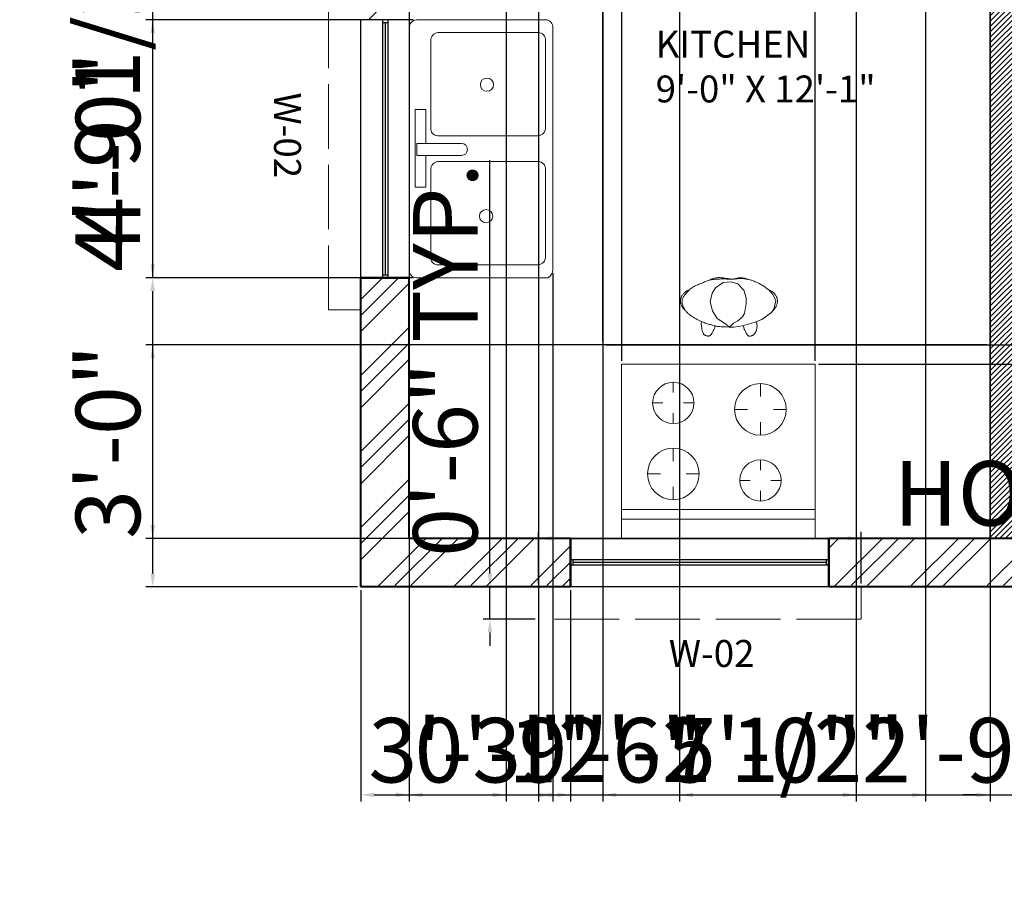
# Model space of a CAD drawing. Units: inches. Extents: x 2386 to 3029, y 792 to 1465.
# Tile 1 of 12: x 2408 to 2591, y 792 to 953. Entities that reach past the tile are written whole.
import ezdxf

# ---------------------------------------------------------------- set-up
doc = ezdxf.new("R2010")
doc.units = ezdxf.units.IN
doc.linetypes.add('ACAD_ISO02W100', pattern=[15, 12, -3])
for name, color, linetype, lineweight in [('A-AREA-IDEN', 4, 'Continuous', 25), ('A-DIMS', 1, 'Continuous', 18), ('A-EQPM', 8, 'Continuous', 18), ('A-FLOR-CASE', 6, 'Continuous', 18), ('A-FLOR-FIXT', 9, 'Continuous', 18), ('A-FURN-ENTG', 8, 'Continuous', 13), ('A-TEXT', 4, 'Continuous', 25), ('A-WALL-EXT', 7, 'Continuous', 40), ('A-WALL-INT', 9, 'Continuous', 30), ('A-WALL-PATT', 9, 'Continuous', 13), ('A-WINDOW', 4, 'Continuous', 25), ('A-WINDOW-OVHD', 4, 'ACAD_ISO02W100', 18)]:
    doc.layers.add(name, color=color, linetype=linetype, lineweight=lineweight)
doc.styles.add('ATT', font='romans.shx')
doc.styles.get("Standard").update_dxf_attribs({"font": 'arial.ttf'})
doc.dimstyles.new('ISO-25', dxfattribs={"dimtxt": 12, "dimasz": 2.5, "dimexe": 1.25, "dimexo": 0.625, "dimtad": 1, "dimlunit": 4, "dimtxsty": 'Standard', "dimcen": 2.5, "dimadec": 0, "dimazin": 0, "dimtfac": 1, "dimtmove": 0, "dimatfit": 3, "dimfxl": 1, "dimarcsym": 0})

# ---------------------------------------------------------------- blocks, each defined once
blk = doc.blocks.new('11PRNG01')
at = {"color": 0, "linetype": 'ByBlock'}
for p, q in [((0, 30), (27, 30)), ((0, 0), (0, 30)), ((3, 0), (3, 30)), ((4.5, 0), (4.5, 30)), ((27, 30), (27, 0)), ((10, 26), (10, 24)), ((21, 25.2), (21, 23.6)), ((6, 22), (8, 22)), ((14, 22), (12, 22)), ((17.8, 22), (19.4, 22)), ((24.2, 22), (22.6, 22)), ((10, 18), (10, 20)), ((21, 18.8), (21, 20.4)), ((20, 12.5), (20, 10.5)), ((9, 11.7), (9, 10.1)), ((5.8, 8.5), (7.4, 8.5)), ((12.2, 8.5), (10.6, 8.5)), ((16, 8.5), (18, 8.5)), ((24, 8.5), (22, 8.5)), ((9, 5.3), (9, 6.9)), ((20, 4.5), (20, 6.5)), ((27, 0), (0, 0))]:
    blk.add_line(p, q, dxfattribs=at)
for centre, radius in [((10, 22), 4), ((21, 22), 3.2), ((20, 8.5), 4), ((9, 8.5), 3.2)]:
    blk.add_circle(centre, radius, dxfattribs=at)
at = {"color": 0, "linetype": 'ByBlock', "style": 'ATT'}
for tag, p, flags in [('ITEM', (0, -11), 3), ('ROOM_NUMBER', (0, -20), 1), ('DEPTH', (0, -29), 3), ('WIDTH', (0, -38), 3)]:
    blk.add_attdef(tag, p, '', height=6, dxfattribs=dict(at, flags=flags))
blk = doc.blocks.new('PERSON-STANDING-PLAN')
for p, q in [((2.26, 9.11), (2.39, 9.19)), ((2.39, 9.19), (2.54, 9.27)), ((2.54, 9.27), (2.7, 9.35)), ((2.7, 9.35), (2.86, 9.42)), ((2.86, 9.42), (3.04, 9.5)), ((3.04, 9.5), (3.21, 9.57)), ((3.21, 9.57), (3.39, 9.65)), ((3.39, 9.65), (3.58, 9.72)), ((3.58, 9.72), (3.76, 9.79)), ((3.76, 9.79), (3.94, 9.87)), ((3.94, 9.87), (4.11, 9.95)), ((4.11, 9.95), (4.28, 10.02)), ((4.28, 10.02), (4.45, 10.1)), ((4.45, 10.1), (4.62, 10.18)), ((4.62, 10.18), (4.79, 10.25)), ((4.79, 10.25), (4.96, 10.31)), ((4.96, 10.31), (5.14, 10.38)), ((5.14, 10.38), (5.33, 10.43)), ((5.33, 10.43), (5.53, 10.48)), ((5.48, 10.5), (5.36, 10.44)), ((5.69, 10.59), (5.48, 10.5)), ((5.53, 10.48), (5.74, 10.51)), ((5.91, 10.67), (5.69, 10.59)), ((5.74, 10.51), (5.95, 10.55)), ((6.13, 10.74), (5.91, 10.67)), ((5.95, 10.55), (6.17, 10.57)), ((6.35, 10.79), (6.13, 10.74)), ((6.17, 10.57), (6.39, 10.59)), ((6.57, 10.84), (6.35, 10.79)), ((6.39, 10.59), (6.61, 10.61)), ((7.91, 9.98), (6.48, 9.01)), ((6.79, 10.87), (6.57, 10.84)), ((6.61, 10.61), (6.83, 10.62)), ((6.99, 10.89), (6.79, 10.87)), ((6.83, 10.62), (7.05, 10.63)), ((7.18, 10.9), (6.99, 10.89)), ((7.05, 10.63), (7.26, 10.64)), ((7.38, 10.9), (7.18, 10.9)), ((7.26, 10.64), (7.47, 10.65)), ((7.57, 10.88), (7.38, 10.9)), ((7.47, 10.65), (7.68, 10.65)), ((7.78, 10.87), (7.57, 10.88)), ((7.68, 10.65), (7.87, 10.65)), ((7.99, 10.84), (7.78, 10.87)), ((7.87, 10.65), (8.06, 10.65)), ((9.39, 10.13), (7.91, 9.98)), ((8.22, 10.82), (7.99, 10.84)), ((8.06, 10.65), (8.23, 10.65)), ((9.71, 10.64), (8.22, 10.82)), ((8.23, 10.65), (8.39, 10.65)), ((8.39, 10.65), (8.54, 10.64)), ((8.54, 10.64), (8.67, 10.64)), ((8.67, 10.64), (8.78, 10.63)), ((8.78, 10.63), (8.89, 10.62)), ((8.89, 10.62), (8.98, 10.61)), ((8.98, 10.61), (9.08, 10.6)), ((9.08, 10.6), (9.16, 10.59)), ((9.16, 10.59), (9.25, 10.59)), ((9.25, 10.59), (9.35, 10.59)), ((9.35, 10.59), (9.44, 10.59)), ((10.63, 9.72), (9.39, 10.13)), ((9.44, 10.59), (9.55, 10.6)), ((9.55, 10.6), (9.66, 10.61)), ((9.9, 10.69), (9.56, 10.61)), ((9.66, 10.61), (9.78, 10.62)), ((9.78, 10.62), (9.9, 10.63)), ((10.22, 10.76), (9.9, 10.69)), ((9.9, 10.63), (10.03, 10.64)), ((10.03, 10.64), (10.16, 10.66)), ((10.16, 10.66), (10.3, 10.67)), ((10.5, 10.81), (10.22, 10.76)), ((10.3, 10.67), (10.45, 10.68)), ((10.45, 10.68), (10.61, 10.7)), ((10.76, 10.84), (10.5, 10.81)), ((10.61, 10.7), (10.76, 10.71)), ((11.79, 8.58), (10.63, 9.72)), ((10.99, 10.86), (10.76, 10.84)), ((10.76, 10.71), (10.92, 10.71)), ((10.92, 10.71), (11.09, 10.72)), ((11.2, 10.87), (10.99, 10.86)), ((11.09, 10.72), (11.25, 10.72)), ((11.4, 10.86), (11.2, 10.87)), ((11.25, 10.72), (11.41, 10.72)), ((11.58, 10.84), (11.4, 10.86)), ((11.41, 10.72), (11.57, 10.71)), ((11.57, 10.71), (11.73, 10.7)), ((11.76, 10.81), (11.58, 10.84)), ((11.73, 10.7), (11.89, 10.68)), ((11.93, 10.77), (11.76, 10.81)), ((11.89, 10.68), (12.04, 10.67)), ((12.11, 10.73), (11.93, 10.77)), ((12.04, 10.67), (12.19, 10.64)), ((12.29, 10.67), (12.11, 10.73)), ((12.19, 10.64), (12.34, 10.62)), ((12.48, 10.61), (12.29, 10.67)), ((12.34, 10.62), (12.48, 10.59)), ((12.68, 10.55), (12.48, 10.61)), ((12.48, 10.59), (12.63, 10.56)), ((12.63, 10.56), (12.77, 10.53)), ((12.91, 10.49), (12.68, 10.55)), ((12.77, 10.53), (12.91, 10.49)), ((12.91, 10.49), (13.05, 10.45)), ((13.17, 10.43), (12.91, 10.49)), ((13.05, 10.45), (13.2, 10.41)), ((13.2, 10.41), (13.35, 10.36)), ((13.35, 10.36), (13.51, 10.3)), ((13.51, 10.3), (13.69, 10.22)), ((13.69, 10.22), (13.89, 10.14)), ((13.89, 10.14), (14.11, 10.04)), ((14.11, 10.04), (14.35, 9.93)), ((14.35, 9.93), (14.61, 9.79)), ((14.61, 9.79), (14.89, 9.64)), ((14.89, 9.64), (15.18, 9.47)), ((15.18, 9.47), (15.49, 9.28)), ((15.49, 9.28), (15.8, 9.07)), ((0.15, 7.32), (0.11, 7.23)), ((0.2, 7.42), (0.15, 7.32)), ((0.25, 7.51), (0.2, 7.42)), ((0.32, 7.61), (0.25, 7.51)), ((0.39, 7.71), (0.32, 7.61)), ((0.48, 7.82), (0.39, 7.71)), ((0.57, 7.92), (0.48, 7.82)), ((0.52, 7.3), (0.6, 7.41)), ((0.67, 8.02), (0.57, 7.92)), ((0.6, 7.41), (0.68, 7.53)), ((0.77, 8.12), (0.67, 8.02)), ((0.68, 7.53), (0.76, 7.64)), ((0.76, 7.64), (0.85, 7.75)), ((0.87, 8.21), (0.77, 8.12)), ((0.85, 7.75), (0.94, 7.85)), ((0.97, 8.29), (0.87, 8.21)), ((0.94, 7.85), (1.03, 7.96)), ((1.08, 8.36), (0.97, 8.29)), ((1.03, 7.96), (1.12, 8.07)), ((1.17, 8.42), (1.08, 8.36)), ((1.12, 8.07), (1.21, 8.17)), ((1.26, 8.47), (1.17, 8.42)), ((1.21, 8.17), (1.3, 8.27)), ((1.35, 8.51), (1.26, 8.47)), ((1.3, 8.27), (1.39, 8.37)), ((1.43, 8.54), (1.35, 8.51)), ((1.39, 8.37), (1.49, 8.47)), ((1.49, 8.56), (1.43, 8.54)), ((1.55, 8.58), (1.49, 8.56)), ((1.49, 8.47), (1.59, 8.57)), ((1.59, 8.59), (1.55, 8.58)), ((1.59, 8.57), (1.69, 8.66)), ((1.62, 8.6), (1.59, 8.59)), ((1.69, 8.66), (1.79, 8.76)), ((1.79, 8.76), (1.9, 8.85)), ((1.9, 8.85), (2.01, 8.94)), ((2.01, 8.94), (2.13, 9.02)), ((2.13, 9.02), (2.26, 9.11)), ((5.88, 8.02), (5.48, 6.38)), ((6.48, 9.01), (5.88, 8.02)), ((12.18, 7.14), (11.79, 8.58)), ((15.8, 9.07), (16.12, 8.84)), ((16.12, 8.84), (16.44, 8.59)), ((16.26, 8.74), (17.17, 7.78)), ((16.44, 8.59), (16.61, 8.53)), ((16.61, 8.53), (16.77, 8.45)), ((16.77, 8.45), (16.94, 8.35)), ((16.94, 8.35), (17.1, 8.23)), ((17.1, 8.23), (17.25, 8.1)), ((17.17, 7.78), (17.68, 6.58)), ((17.25, 8.1), (17.38, 7.96)), ((17.38, 7.96), (17.51, 7.82)), ((17.51, 7.82), (17.61, 7.69)), ((17.61, 7.69), (17.7, 7.56)), ((17.7, 7.56), (17.78, 7.45)), ((17.78, 7.45), (17.84, 7.34)), ((17.84, 7.34), (17.88, 7.24)), ((0.01, 6.79), (0, 6.7)), ((0, 6.7), (0, 6.61)), ((0, 6.61), (0, 6.52)), ((0, 6.52), (0, 6.42)), ((0, 6.42), (0.01, 6.33)), ((0.02, 6.88), (0.01, 6.79)), ((0.01, 6.33), (0.02, 6.22)), ((0.04, 6.97), (0.02, 6.88)), ((0.02, 6.22), (0.04, 6.12)), ((0.06, 7.06), (0.04, 6.97)), ((0.04, 6.12), (0.06, 6)), ((0.08, 7.15), (0.06, 7.06)), ((0.06, 6), (0.1, 5.88)), ((0.11, 7.23), (0.08, 7.15)), ((0.1, 5.88), (0.15, 5.75)), ((0.15, 5.75), (0.23, 5.6)), ((0.23, 5.6), (0.33, 5.43)), ((0.28, 6.52), (0.29, 6.66)), ((0.29, 6.38), (0.28, 6.52)), ((0.29, 6.66), (0.31, 6.8)), ((0.3, 6.24), (0.29, 6.38)), ((0.32, 6.09), (0.3, 6.24)), ((0.31, 6.8), (0.35, 6.93)), ((0.35, 5.95), (0.32, 6.09)), ((0.35, 6.93), (0.4, 7.06)), ((0.39, 5.81), (0.35, 5.95)), ((0.43, 5.68), (0.39, 5.81)), ((0.4, 7.06), (0.46, 7.18)), ((0.48, 5.55), (0.43, 5.68)), ((0.46, 7.18), (0.52, 7.3)), ((0.53, 5.42), (0.48, 5.55)), ((5.48, 6.38), (5.95, 4.72)), ((11.9, 4.25), (12.22, 6.07)), ((12.22, 6.07), (12.18, 7.14)), ((17.68, 6.58), (17.36, 5.01)), ((17.78, 5.6), (17.68, 5.42)), ((17.86, 5.75), (17.78, 5.6)), ((17.91, 5.88), (17.86, 5.75)), ((17.88, 7.24), (17.92, 7.15)), ((17.94, 6), (17.91, 5.88)), ((17.92, 7.15), (17.95, 7.06)), ((17.96, 6.12), (17.94, 6)), ((17.95, 7.06), (17.97, 6.97)), ((17.98, 6.22), (17.96, 6.12)), ((17.97, 6.97), (17.98, 6.88)), ((17.98, 6.88), (17.99, 6.79)), ((17.99, 6.33), (17.98, 6.22)), ((17.99, 6.79), (18, 6.7)), ((18, 6.42), (17.99, 6.33)), ((18, 6.7), (18.01, 6.61)), ((18.01, 6.52), (18, 6.42)), ((18.01, 6.61), (18.01, 6.52)), ((0.33, 5.43), (0.48, 5.23)), ((0.48, 5.23), (0.67, 5.01)), ((0.58, 5.3), (0.53, 5.42)), ((0.64, 5.19), (0.58, 5.3)), ((0.7, 5.07), (0.64, 5.19)), ((0.67, 5.01), (0.91, 4.75)), ((0.77, 4.96), (0.7, 5.07)), ((0.85, 4.85), (0.77, 4.96)), ((0.93, 4.74), (0.85, 4.85)), ((1.01, 4.63), (0.93, 4.74)), ((1.1, 4.52), (1.01, 4.63)), ((1.21, 4.41), (1.1, 4.52)), ((1.32, 4.3), (1.21, 4.41)), ((1.44, 4.19), (1.32, 4.3)), ((1.57, 4.08), (1.44, 4.19)), ((1.72, 3.96), (1.57, 4.08)), ((1.88, 3.84), (1.72, 3.96)), ((2.06, 3.71), (1.88, 3.84)), ((2.26, 3.59), (2.06, 3.71)), ((5.95, 4.72), (6.81, 3.29)), ((11.44, 3.53), (11.9, 4.25)), ((16.88, 4.4), (15.08, 3.08)), ((17.36, 5.01), (16.88, 4.4)), ((17.37, 5), (17.14, 4.74)), ((17.54, 5.23), (17.37, 5)), ((17.68, 5.42), (17.54, 5.23)), ((2.46, 3.46), (2.26, 3.59)), ((2.67, 3.34), (2.46, 3.46)), ((2.89, 3.21), (2.67, 3.34)), ((3.11, 3.09), (2.89, 3.21)), ((3.33, 2.98), (3.11, 3.09)), ((3.56, 2.87), (3.33, 2.98)), ((3.77, 2.77), (3.56, 2.87)), ((3.99, 2.68), (3.77, 2.77)), ((3.86, 2.7), (3.84, 2.5)), ((3.84, 2.5), (3.84, 2.27)), ((3.84, 2.27), (3.86, 2.03)), ((3.86, 2.03), (3.89, 1.79)), ((4.2, 2.6), (3.99, 2.68)), ((4.4, 2.52), (4.2, 2.6)), ((4.6, 2.45), (4.4, 2.52)), ((4.8, 2.38), (4.6, 2.45)), ((5, 2.32), (4.8, 2.38)), ((5.19, 2.26), (5, 2.32)), ((5.38, 2.2), (5.19, 2.26)), ((5.56, 2.15), (5.38, 2.2)), ((5.74, 2.09), (5.56, 2.15)), ((5.92, 2.05), (5.74, 2.09)), ((6.09, 2), (5.92, 2.05)), ((6.25, 1.96), (6.09, 2)), ((6.41, 1.92), (6.25, 1.96)), ((6.36, 1.65), (6.46, 1.91)), ((6.55, 1.89), (6.41, 1.92)), ((6.7, 1.86), (6.55, 1.89)), ((6.85, 1.83), (6.7, 1.86)), ((6.81, 3.29), (8.17, 2.41)), ((7.04, 1.81), (6.85, 1.83)), ((8.17, 2.41), (9.1, 1.71)), ((9.1, 1.71), (9.82, 2.41)), ((9.82, 2.41), (10.66, 2.88)), ((11.53, 1.95), (9.89, 1.71)), ((10.66, 2.88), (11.44, 3.53)), ((13.68, 2.54), (11.53, 1.95)), ((11.63, 1.91), (11.75, 1.61)), ((15.08, 3.08), (13.68, 2.54)), ((14.17, 2.51), (14.14, 2.7)), ((14.19, 2.34), (14.17, 2.51)), ((14.2, 2.16), (14.19, 2.34)), ((14.21, 1.99), (14.2, 2.16)), ((14.2, 1.68), (14.21, 1.83)), ((14.21, 1.83), (14.21, 1.99)), ((3.89, 1.79), (3.93, 1.54)), ((3.93, 1.54), (3.98, 1.3)), ((3.98, 1.3), (4.03, 1.08)), ((4.03, 1.08), (4.09, 0.89)), ((4.09, 0.89), (4.14, 0.73)), ((4.14, 0.73), (4.19, 0.59)), ((4.19, 0.59), (4.24, 0.49)), ((4.24, 0.49), (4.29, 0.4)), ((4.29, 0.4), (4.34, 0.34)), ((4.34, 0.34), (4.39, 0.28)), ((4.39, 0.28), (4.45, 0.24)), ((4.45, 0.24), (4.51, 0.2)), ((4.51, 0.2), (4.57, 0.17)), ((4.57, 0.17), (4.64, 0.14)), ((4.64, 0.14), (4.72, 0.11)), ((4.72, 0.11), (4.79, 0.09)), ((4.79, 0.09), (4.86, 0.07)), ((4.86, 0.07), (4.93, 0.05)), ((4.93, 0.05), (5, 0.04)), ((5, 0.04), (5.07, 0.03)), ((5.07, 0.03), (5.13, 0.03)), ((5.13, 0.03), (5.19, 0.03)), ((5.19, 0.03), (5.24, 0.03)), ((5.24, 0.03), (5.29, 0.04)), ((5.29, 0.04), (5.34, 0.05)), ((5.34, 0.05), (5.39, 0.06)), ((5.39, 0.06), (5.43, 0.08)), ((5.43, 0.08), (5.47, 0.11)), ((5.47, 0.11), (5.51, 0.13)), ((5.51, 0.13), (5.55, 0.16)), ((5.55, 0.16), (5.59, 0.2)), ((5.59, 0.2), (5.63, 0.24)), ((5.63, 0.24), (5.68, 0.29)), ((5.68, 0.29), (5.72, 0.35)), ((5.72, 0.35), (5.77, 0.42)), ((5.77, 0.42), (5.82, 0.5)), ((5.82, 0.5), (5.88, 0.59)), ((5.88, 0.59), (5.94, 0.7)), ((5.94, 0.7), (6.01, 0.83)), ((6.01, 0.83), (6.09, 0.99)), ((6.09, 0.99), (6.17, 1.17)), ((6.17, 1.17), (6.26, 1.39)), ((6.26, 1.39), (6.36, 1.65)), ((7.27, 1.79), (7.04, 1.81)), ((7.57, 1.77), (7.27, 1.79)), ((7.97, 1.75), (7.57, 1.77)), ((8.47, 1.73), (7.97, 1.75)), ((9.1, 1.71), (8.47, 1.73)), ((9.89, 1.71), (9.1, 1.71)), ((11.75, 1.61), (11.85, 1.34)), ((11.85, 1.34), (11.95, 1.1)), ((11.95, 1.1), (12.05, 0.89)), ((12.05, 0.89), (12.13, 0.71)), ((12.13, 0.71), (12.22, 0.55)), ((12.22, 0.55), (12.29, 0.41)), ((12.29, 0.41), (12.37, 0.3)), ((12.37, 0.3), (12.44, 0.21)), ((12.44, 0.21), (12.51, 0.14)), ((12.51, 0.14), (12.58, 0.08)), ((12.58, 0.08), (12.64, 0.04)), ((12.64, 0.04), (12.71, 0.02)), ((12.71, 0.02), (12.77, 0)), ((12.77, 0), (12.84, 0)), ((12.84, 0), (12.9, 0)), ((12.9, 0), (12.97, 0.01)), ((12.97, 0.01), (13.03, 0.02)), ((13.03, 0.02), (13.1, 0.04)), ((13.1, 0.04), (13.17, 0.06)), ((13.17, 0.06), (13.24, 0.09)), ((13.24, 0.09), (13.3, 0.12)), ((13.3, 0.12), (13.37, 0.15)), ((13.37, 0.15), (13.43, 0.18)), ((13.43, 0.18), (13.49, 0.22)), ((13.49, 0.22), (13.55, 0.26)), ((13.55, 0.26), (13.61, 0.31)), ((13.61, 0.31), (13.67, 0.35)), ((13.67, 0.35), (13.72, 0.41)), ((13.72, 0.41), (13.77, 0.47)), ((13.77, 0.47), (13.82, 0.53)), ((13.82, 0.53), (13.87, 0.6)), ((13.87, 0.6), (13.92, 0.67)), ((13.92, 0.67), (13.96, 0.75)), ((13.96, 0.75), (14.01, 0.84)), ((14.01, 0.84), (14.05, 0.94)), ((14.05, 0.94), (14.08, 1.04)), ((14.08, 1.04), (14.12, 1.15)), ((14.12, 1.15), (14.14, 1.27)), ((14.14, 1.27), (14.17, 1.4)), ((14.17, 1.4), (14.19, 1.54)), ((14.19, 1.54), (14.2, 1.68))]:
    blk.add_line(p, q)
blk = doc.blocks.new('WINDOW-48IN')
for p, q in [((0, 9), (48, 9)), ((0, 0), (0, 9)), ((48, 9), (48, 0)), ((48, 5), (0, 5)), ((48, 4), (0, 4)), ((0.5, 4), (0.5, 5)), ((47.5, 4.5), (0.5, 4.5)), ((47.5, 5), (47.5, 4)), ((48, 0), (0, 0))]:
    blk.add_line(p, q)
blk = doc.blocks.new('WINDOW-HOOD-48IN')
for p, q in [((0, 0), (0, 6)), ((60, 6), (60, 0)), ((60, 0), (0, 0))]:
    blk.add_line(p, q)
blk = doc.blocks.new('*D42')
at = {"layer": 'A-DIMS', "color": 0, "lineweight": -2, "transparency": 16777216}
for p, q in [((2504.19, 848.57), (2504.19, 858.2)), ((2506.69, 856.95), (2561.69, 856.95)), ((2564.19, 848.57), (2564.19, 858.2)), ((2564.19, 856.95), (2740.1, 856.95))]:
    blk.add_line(p, q, dxfattribs=at)
at = {"layer": 'A-DIMS', "color": 0, "transparency": 16777216}
for points in [[(2506.69, 857.36), (2506.69, 856.53), (2504.19, 856.95)], [(2561.69, 857.36), (2561.69, 856.53), (2564.19, 856.95)]]:
    blk.add_solid(points, dxfattribs=at)
at = {"layer": 'Defpoints', "color": 0, "transparency": 16777216}
for p in [(2564.19, 856.95), (2504.19, 847.95), (2564.19, 847.95)]:
    blk.add_point(p, dxfattribs=at)
at = {"layer": 'A-DIMS', "color": 0, "transparency": 16777216, "insert": (2653.39, 863.78), "char_height": 12, "attachment_point": 5}
blk.add_mtext('HOOD W-02 5\'-0" TYP.', dxfattribs=at)
blk = doc.blocks.new('*D43')
at = {"layer": 'A-DIMS', "color": 0, "lineweight": -2, "transparency": 16777216}
for p, q in [((2495.19, 850.45), (2495.19, 927.34)), ((2503.57, 847.95), (2493.94, 847.95)), ((2495.19, 841.95), (2495.19, 847.95)), ((2503.57, 841.95), (2493.94, 841.95)), ((2495.19, 839.45), (2495.19, 836.95))]:
    blk.add_line(p, q, dxfattribs=at)
at = {"layer": 'A-DIMS', "color": 0, "transparency": 16777216}
for points in [[(2494.77, 850.45), (2495.61, 850.45), (2495.19, 847.95)], [(2494.77, 839.45), (2495.61, 839.45), (2495.19, 841.95)]]:
    blk.add_solid(points, dxfattribs=at)
at = {"layer": 'Defpoints', "color": 0, "transparency": 16777216}
for p in [(2495.19, 847.95), (2504.19, 847.95), (2504.19, 841.95)]:
    blk.add_point(p, dxfattribs=at)
at = {"layer": 'A-DIMS', "color": 0, "transparency": 16777216, "insert": (2488.44, 890.15), "char_height": 12, "attachment_point": 5, "rotation": 90}
blk.add_mtext('0\'-6" TYP.', dxfattribs=at)
blk = doc.blocks.new('*D60')
at = {"layer": 'A-DIMS', "color": 0, "lineweight": -2, "transparency": 16777216}
for p, q in [((2471.19, 847.32), (2471.19, 808)), ((2510.19, 847.32), (2510.19, 808)), ((2473.69, 809.25), (2507.69, 809.25))]:
    blk.add_line(p, q, dxfattribs=at)
at = {"layer": 'A-DIMS', "color": 0, "transparency": 16777216}
for points in [[(2473.69, 809.66), (2473.69, 808.83), (2471.19, 809.25)], [(2507.69, 809.66), (2507.69, 808.83), (2510.19, 809.25)]]:
    blk.add_solid(points, dxfattribs=at)
at = {"layer": 'Defpoints', "color": 0, "transparency": 16777216}
for p in [(2471.19, 847.95), (2510.19, 847.95), (2510.19, 809.25)]:
    blk.add_point(p, dxfattribs=at)
at = {"layer": 'A-DIMS', "color": 0, "transparency": 16777216, "insert": (2490.69, 816), "char_height": 12, "attachment_point": 5}
blk.add_mtext('3\'-3"', dxfattribs=at)
blk = doc.blocks.new('*D61')
at = {"layer": 'A-DIMS', "color": 0, "lineweight": -2, "transparency": 16777216}
for p, q in [((2432.49, 905.45), (2432.49, 969.54)), ((2470.57, 905.45), (2431.24, 905.45)), ((2432.49, 850.45), (2432.49, 902.95)), ((2470.57, 847.95), (2431.24, 847.95))]:
    blk.add_line(p, q, dxfattribs=at)
at = {"layer": 'A-DIMS', "color": 0, "transparency": 16777216}
for points in [[(2432.07, 902.95), (2432.91, 902.95), (2432.49, 905.45)], [(2432.07, 850.45), (2432.91, 850.45), (2432.49, 847.95)]]:
    blk.add_solid(points, dxfattribs=at)
at = {"layer": 'Defpoints', "color": 0, "transparency": 16777216}
for p in [(2432.49, 905.45), (2471.19, 905.45), (2471.19, 847.95)]:
    blk.add_point(p, dxfattribs=at)
at = {"layer": 'A-DIMS', "color": 0, "transparency": 16777216, "insert": (2425.66, 938.74), "char_height": 12, "attachment_point": 5, "rotation": 90}
blk.add_mtext('4\'-9 1/2"', dxfattribs=at)
blk = doc.blocks.new('*D71')
at = {"layer": 'A-DIMS', "color": 0, "lineweight": -2, "transparency": 16777216}
for p, q in [((2480.19, 856.32), (2480.19, 808)), ((2471.19, 847.32), (2471.19, 808)), ((2473.69, 809.25), (2477.69, 809.25)), ((2480.19, 809.25), (2515.84, 809.25))]:
    blk.add_line(p, q, dxfattribs=at)
at = {"layer": 'A-DIMS', "color": 0, "transparency": 16777216}
for points in [[(2473.69, 809.66), (2473.69, 808.83), (2471.19, 809.25)], [(2477.69, 809.66), (2477.69, 808.83), (2480.19, 809.25)]]:
    blk.add_solid(points, dxfattribs=at)
at = {"layer": 'Defpoints', "color": 0, "transparency": 16777216}
for p in [(2480.19, 856.95), (2471.19, 847.95), (2480.19, 809.25)]:
    blk.add_point(p, dxfattribs=at)
at = {"layer": 'A-DIMS', "color": 0, "transparency": 16777216, "insert": (2499.26, 816), "char_height": 12, "attachment_point": 5}
blk.add_mtext('0\'-9"', dxfattribs=at)
blk = doc.blocks.new('*D72')
at = {"layer": 'A-DIMS', "color": 0, "lineweight": -2, "transparency": 16777216}
for p, q in [((2588.19, 856.32), (2588.19, 808)), ((2594.19, 847.32), (2594.19, 808)), ((2585.69, 809.25), (2583.19, 809.25)), ((2588.19, 809.25), (2594.19, 809.25)), ((2596.69, 809.25), (2632.34, 809.25))]:
    blk.add_line(p, q, dxfattribs=at)
at = {"layer": 'A-DIMS', "color": 0, "transparency": 16777216}
for points in [[(2585.69, 809.66), (2585.69, 808.83), (2588.19, 809.25)], [(2596.69, 809.66), (2596.69, 808.83), (2594.19, 809.25)]]:
    blk.add_solid(points, dxfattribs=at)
at = {"layer": 'Defpoints', "color": 0, "transparency": 16777216}
for p in [(2588.19, 856.95), (2594.19, 847.95), (2594.19, 809.25)]:
    blk.add_point(p, dxfattribs=at)
at = {"layer": 'A-DIMS', "color": 0, "transparency": 16777216, "insert": (2615.76, 816), "char_height": 12, "attachment_point": 5}
blk.add_mtext('0\'-6"', dxfattribs=at)
blk = doc.blocks.new('*D73')
at = {"layer": 'A-DIMS', "color": 0, "lineweight": -2, "transparency": 16777216}
for p, q in [((2519.68, 889.97), (2519.68, 1427.9)), ((2555.68, 889.97), (2555.68, 1427.9)), ((2522.18, 1426.65), (2553.18, 1426.65))]:
    blk.add_line(p, q, dxfattribs=at)
at = {"layer": 'A-DIMS', "color": 0, "transparency": 16777216}
for points in [[(2522.18, 1427.06), (2522.18, 1426.23), (2519.68, 1426.65)], [(2553.18, 1427.06), (2553.18, 1426.23), (2555.68, 1426.65)]]:
    blk.add_solid(points, dxfattribs=at)
at = {"layer": 'Defpoints', "color": 0, "transparency": 16777216}
for p in [(2555.68, 1426.65), (2519.68, 889.35), (2555.68, 889.35)]:
    blk.add_point(p, dxfattribs=at)
at = {"layer": 'A-DIMS', "color": 0, "transparency": 16777216, "insert": (2537.68, 1433.4), "char_height": 12, "attachment_point": 5}
blk.add_mtext('3\'-0"', dxfattribs=at)
blk = doc.blocks.new('*D74')
at = {"layer": 'A-DIMS', "color": 0, "lineweight": -2, "transparency": 16777216}
for p, q in [((2556.3, 889.35), (2931.14, 889.35)), ((2929.89, 886.85), (2929.89, 859.45)), ((2556.3, 856.95), (2931.14, 856.95)), ((2929.89, 856.95), (2929.89, 793.13))]:
    blk.add_line(p, q, dxfattribs=at)
at = {"layer": 'A-DIMS', "color": 0, "transparency": 16777216}
for points in [[(2929.47, 886.85), (2930.31, 886.85), (2929.89, 889.35)], [(2929.47, 859.45), (2930.31, 859.45), (2929.89, 856.95)]]:
    blk.add_solid(points, dxfattribs=at)
at = {"layer": 'Defpoints', "color": 0, "transparency": 16777216}
for p in [(2555.68, 889.35), (2555.68, 856.95), (2929.89, 856.95)]:
    blk.add_point(p, dxfattribs=at)
at = {"layer": 'A-DIMS', "color": 0, "transparency": 16777216, "insert": (2923.06, 823.79), "char_height": 12, "attachment_point": 5, "rotation": 90}
blk.add_mtext('2\'-8 1/2"', dxfattribs=at)
blk = doc.blocks.new('*D76')
at = {"layer": 'A-DIMS', "color": 0, "lineweight": -2, "transparency": 16777216}
for p, q in [((2480.19, 1174.77), (2480.19, 808)), ((2498.19, 1174.77), (2498.19, 808)), ((2482.69, 809.25), (2495.69, 809.25)), ((2498.19, 809.25), (2532.71, 809.25))]:
    blk.add_line(p, q, dxfattribs=at)
at = {"layer": 'A-DIMS', "color": 0, "transparency": 16777216}
for points in [[(2482.69, 809.66), (2482.69, 808.83), (2480.19, 809.25)], [(2495.69, 809.66), (2495.69, 808.83), (2498.19, 809.25)]]:
    blk.add_solid(points, dxfattribs=at)
at = {"layer": 'Defpoints', "color": 0, "transparency": 16777216}
for p in [(2480.19, 1175.39), (2498.19, 1175.39), (2498.19, 809.25)]:
    blk.add_point(p, dxfattribs=at)
at = {"layer": 'A-DIMS', "color": 0, "transparency": 16777216, "insert": (2516.7, 816), "char_height": 12, "attachment_point": 5}
blk.add_mtext('1\'-6"', dxfattribs=at)
blk = doc.blocks.new('*D77')
at = {"layer": 'A-DIMS', "color": 0, "lineweight": -2, "transparency": 16777216}
for p, q in [((2516.19, 1103.32), (2516.19, 808)), ((2576.19, 1103.32), (2576.19, 808)), ((2518.69, 809.25), (2573.69, 809.25))]:
    blk.add_line(p, q, dxfattribs=at)
at = {"layer": 'A-DIMS', "color": 0, "transparency": 16777216}
for points in [[(2518.69, 809.66), (2518.69, 808.83), (2516.19, 809.25)], [(2573.69, 809.66), (2573.69, 808.83), (2576.19, 809.25)]]:
    blk.add_solid(points, dxfattribs=at)
at = {"layer": 'Defpoints', "color": 0, "transparency": 16777216}
for p in [(2516.19, 1103.95), (2576.19, 1103.95), (2576.19, 809.25)]:
    blk.add_point(p, dxfattribs=at)
at = {"layer": 'A-DIMS', "color": 0, "transparency": 16777216, "insert": (2546.19, 816), "char_height": 12, "attachment_point": 5}
blk.add_mtext('5\'-0"', dxfattribs=at)
blk = doc.blocks.new('*D94')
at = {"layer": 'A-DIMS', "color": 0, "lineweight": -2, "transparency": 16777216}
for p, q in [((2504.19, 1205.32), (2504.19, 808)), ((2588.19, 1205.32), (2588.19, 808)), ((2506.69, 809.25), (2585.69, 809.25))]:
    blk.add_line(p, q, dxfattribs=at)
at = {"layer": 'A-DIMS', "color": 0, "transparency": 16777216}
for points in [[(2506.69, 809.66), (2506.69, 808.83), (2504.19, 809.25)], [(2585.69, 809.66), (2585.69, 808.83), (2588.19, 809.25)]]:
    blk.add_solid(points, dxfattribs=at)
at = {"layer": 'Defpoints', "color": 0, "transparency": 16777216}
for p in [(2504.19, 1205.95), (2588.19, 1205.95), (2588.19, 809.25)]:
    blk.add_point(p, dxfattribs=at)
at = {"layer": 'A-DIMS', "color": 0, "transparency": 16777216, "insert": (2546.19, 816), "char_height": 12, "attachment_point": 5}
blk.add_mtext('7\'-0"', dxfattribs=at)
blk = doc.blocks.new('*D96')
at = {"layer": 'A-DIMS', "color": 0, "lineweight": -2, "transparency": 16777216}
for p, q in [((2516.19, 893.57), (2516.19, 1427.9)), ((2588.19, 893.57), (2588.19, 1427.9)), ((2518.69, 1426.65), (2585.69, 1426.65))]:
    blk.add_line(p, q, dxfattribs=at)
at = {"layer": 'A-DIMS', "color": 0, "transparency": 16777216}
for points in [[(2518.69, 1427.06), (2518.69, 1426.23), (2516.19, 1426.65)], [(2585.69, 1427.06), (2585.69, 1426.23), (2588.19, 1426.65)]]:
    blk.add_solid(points, dxfattribs=at)
at = {"layer": 'Defpoints', "color": 0, "transparency": 16777216}
for p in [(2588.19, 1426.65), (2516.19, 892.95), (2588.19, 892.95)]:
    blk.add_point(p, dxfattribs=at)
at = {"layer": 'A-DIMS', "color": 0, "transparency": 16777216, "insert": (2552.19, 1433.4), "char_height": 12, "attachment_point": 5}
blk.add_mtext('6\'-0"', dxfattribs=at)
blk = doc.blocks.new('*D97')
at = {"layer": 'A-DIMS', "color": 0, "lineweight": -2, "transparency": 16777216}
for p, q in [((2516.82, 965.95), (2931.14, 965.95)), ((2929.89, 895.45), (2929.89, 963.45)), ((2516.82, 892.95), (2931.14, 892.95))]:
    blk.add_line(p, q, dxfattribs=at)
at = {"layer": 'A-DIMS', "color": 0, "transparency": 16777216}
for points in [[(2929.47, 963.45), (2930.31, 963.45), (2929.89, 965.95)], [(2929.47, 895.45), (2930.31, 895.45), (2929.89, 892.95)]]:
    blk.add_solid(points, dxfattribs=at)
at = {"layer": 'Defpoints', "color": 0, "transparency": 16777216}
for p in [(2516.19, 965.95), (2929.89, 965.95), (2516.19, 892.95)]:
    blk.add_point(p, dxfattribs=at)
at = {"layer": 'A-DIMS', "color": 0, "transparency": 16777216, "insert": (2923.14, 929.45), "char_height": 12, "attachment_point": 5, "rotation": 90}
blk.add_mtext('6\'-1"', dxfattribs=at)
blk = doc.blocks.new('*D98')
at = {"layer": 'A-DIMS', "color": 0, "lineweight": -2, "transparency": 16777216}
for p, q in [((2587.57, 892.95), (2431.24, 892.95)), ((2432.49, 859.45), (2432.49, 890.45)), ((2587.57, 856.95), (2431.24, 856.95))]:
    blk.add_line(p, q, dxfattribs=at)
at = {"layer": 'A-DIMS', "color": 0, "transparency": 16777216}
for points in [[(2432.07, 890.45), (2432.91, 890.45), (2432.49, 892.95)], [(2432.07, 859.45), (2432.91, 859.45), (2432.49, 856.95)]]:
    blk.add_solid(points, dxfattribs=at)
at = {"layer": 'Defpoints', "color": 0, "transparency": 16777216}
for p in [(2432.49, 892.95), (2588.19, 892.95), (2588.19, 856.95)]:
    blk.add_point(p, dxfattribs=at)
at = {"layer": 'A-DIMS', "color": 0, "transparency": 16777216, "insert": (2425.73, 874.95), "char_height": 12, "attachment_point": 5, "rotation": 90}
blk.add_mtext('3\'-0"', dxfattribs=at)
blk = doc.blocks.new('*D99')
at = {"layer": 'A-DIMS', "color": 0, "lineweight": -2, "transparency": 16777216}
for p, q in [((2530.41, 1210.29), (2530.41, 808)), ((2563.26, 1210.63), (2563.26, 808)), ((2532.91, 809.25), (2560.76, 809.25)), ((2563.26, 809.25), (2599.11, 809.25))]:
    blk.add_line(p, q, dxfattribs=at)
at = {"layer": 'A-DIMS', "color": 0, "transparency": 16777216}
for points in [[(2532.91, 809.66), (2532.91, 808.83), (2530.41, 809.25)], [(2560.76, 809.66), (2560.76, 808.83), (2563.26, 809.25)]]:
    blk.add_solid(points, dxfattribs=at)
at = {"layer": 'Defpoints', "color": 0, "transparency": 16777216}
for p in [(2530.41, 1210.91), (2563.26, 1211.26), (2563.26, 809.25)]:
    blk.add_point(p, dxfattribs=at)
at = {"layer": 'A-DIMS', "color": 0, "transparency": 16777216, "insert": (2582.43, 816), "char_height": 12, "attachment_point": 5}
blk.add_mtext('2\'-9"', dxfattribs=at)
blk = doc.blocks.new('*D102')
at = {"layer": 'A-DIMS', "color": 0, "lineweight": -2, "transparency": 16777216}
for p, q in [((2480.19, 906.32), (2480.19, 808)), ((2506.86, 906.32), (2506.86, 808)), ((2482.69, 809.25), (2504.36, 809.25)), ((2506.86, 809.25), (2570.67, 809.25))]:
    blk.add_line(p, q, dxfattribs=at)
at = {"layer": 'A-DIMS', "color": 0, "transparency": 16777216}
for points in [[(2482.69, 809.66), (2482.69, 808.83), (2480.19, 809.25)], [(2504.36, 809.66), (2504.36, 808.83), (2506.86, 809.25)]]:
    blk.add_solid(points, dxfattribs=at)
at = {"layer": 'Defpoints', "color": 0, "transparency": 16777216}
for p in [(2480.19, 906.95), (2506.86, 906.95), (2506.86, 809.25)]:
    blk.add_point(p, dxfattribs=at)
at = {"layer": 'A-DIMS', "color": 0, "transparency": 16777216, "insert": (2540.01, 816.08), "char_height": 12, "attachment_point": 5}
blk.add_mtext('2\'-2 1/2"', dxfattribs=at)
blk = doc.blocks.new('*D103')
at = {"layer": 'A-DIMS', "color": 0, "lineweight": -2, "transparency": 16777216}
for p, q in [((2480.9, 953.44), (2431.24, 953.44)), ((2432.49, 907.94), (2432.49, 950.94)), ((2480.9, 905.44), (2431.24, 905.44))]:
    blk.add_line(p, q, dxfattribs=at)
at = {"layer": 'A-DIMS', "color": 0, "transparency": 16777216}
for points in [[(2432.07, 950.94), (2432.91, 950.94), (2432.49, 953.44)], [(2432.07, 907.94), (2432.91, 907.94), (2432.49, 905.44)]]:
    blk.add_solid(points, dxfattribs=at)
at = {"layer": 'Defpoints', "color": 0, "transparency": 16777216}
for p in [(2432.49, 953.44), (2481.52, 953.44), (2481.52, 905.44)]:
    blk.add_point(p, dxfattribs=at)
at = {"layer": 'A-DIMS', "color": 0, "transparency": 16777216, "insert": (2425.74, 929.44), "char_height": 12, "attachment_point": 5, "rotation": 90}
blk.add_mtext('4\'-0"', dxfattribs=at)

msp = doc.modelspace()

# ---------------------------------------------------------------- hatches: boundary and pattern name
at = {"layer": 'A-WALL-PATT'}
h = msp.add_hatch(dxfattribs=at)
h.set_pattern_fill('GOST_GROUND', color=256)
h.paths.add_polyline_path([(2480.19, 1276.948), (2471.19, 1276.948), (2471.19, 1211.948), (2480.19, 1211.948)])
h.paths.add_polyline_path([(2480.19, 1378.948), (2510.19, 1378.948), (2510.19, 1378.969), (2523.779, 1378.969), (2580.602, 1378.959), (2580.602, 1378.969), (2594.19, 1378.969), (2642.19, 1378.948), (2642.19, 1387.948), (2471.19, 1387.948), (2471.19, 1336.948), (2480.19, 1336.948)])
h.paths.add_polyline_path([(2891.19, 1387.948), (2666.19, 1387.948), (2666.19, 1378.948), (2882.19, 1378.948), (2882.19, 1355.948), (2891.19, 1355.948)])
h.paths.add_polyline_path([(2891.19, 1331.948), (2882.19, 1331.948), (2882.19, 1331.449), (2882.19, 1261.948), (2891.19, 1261.948)])
h.paths.add_polyline_path([(2891.19, 1201.948), (2882.19, 1201.948), (2882.19, 1189.948), (2882.19, 1159.948), (2882.19, 1117.948), (2891.19, 1117.948)])
h.paths.add_polyline_path([(2891.19, 1057.948), (2882.19, 1057.948), (2882.19, 856.948), (2882.19, 847.948), (2891.19, 847.948)])
h.paths.add_polyline_path([(2594.19, 856.948), (2558.19, 856.948), (2558.19, 847.948), (2594.19, 847.948)])
h.paths.add_polyline_path([(2510.19, 856.948), (2480.19, 856.948), (2480.19, 905.448), (2471.19, 905.448), (2471.19, 847.948), (2510.19, 847.948)])
h.paths.add_polyline_path([(2480.19, 1007.948), (2471.19, 1007.948), (2471.19, 953.448), (2480.19, 953.448)])
h.paths.add_polyline_path([(2480.19, 1103.948), (2471.19, 1103.948), (2471.19, 1043.948), (2480.19, 1043.948)])
h = msp.add_hatch(dxfattribs=at)
h.set_pattern_fill('JIS_WOOD', color=256)
h.paths.add_polyline_path([(2624.19, 1229.948), (2624.19, 1145.948), (2618.19, 1145.948), (2618.19, 1140.548), (2618.19, 1139.948), (2630.19, 1139.948), (2630.19, 1240.948), (2624.19, 1240.948), (2624.19, 1234.948), (2480.19, 1234.948), (2480.19, 1229.948)])
h.paths.add_polyline_path([(2582.19, 1139.948), (2582.19, 1145.948), (2480.19, 1145.948), (2480.19, 1139.948)], flags=17)
h.paths.add_polyline_path([(2480.19, 1007.948), (2480.19, 1001.948), (2546.19, 1001.948), (2546.19, 1007.348), (2546.19, 1007.948)])
h.paths.add_polyline_path([(2594.19, 1007.948), (2582.19, 1007.948), (2582.19, 1001.948), (2588.19, 1001.948), (2588.19, 856.948), (2594.19, 856.948), (2594.19, 914.948), (2606.19, 914.948), (2606.19, 920.948), (2594.19, 920.948)])
h.paths.add_polyline_path([(2738.19, 1015.948), (2882.19, 1015.948), (2882.19, 1021.948), (2738.19, 1021.948), (2738.19, 1111.948), (2732.19, 1111.948), (2732.19, 920.948), (2720.19, 920.948), (2720.19, 914.948), (2732.19, 914.948), (2732.19, 856.948), (2738.19, 856.948)])
h.paths.add_polyline_path([(2660.19, 914.948), (2660.19, 920.948), (2648.19, 920.948), (2648.19, 914.948)])
h.paths.add_polyline_path([(2738.19, 1159.948), (2738.19, 1165.948), (2737.59, 1165.948), (2732.19, 1165.948), (2732.19, 1147.948), (2737.59, 1147.948), (2738.19, 1147.948), (2738.19, 1153.948), (2882.19, 1153.948), (2882.19, 1159.948)])
h.paths.add_polyline_path([(2732.19, 1201.948), (2738.19, 1201.948), (2738.19, 1303.948), (2774.19, 1303.948), (2774.19, 1308.948), (2768.19, 1308.948), (2768.19, 1378.948), (2762.19, 1378.948), (2762.19, 1308.948), (2726.19, 1308.948), (2726.19, 1303.948), (2732.19, 1303.948)])
h.paths.add_polyline_path([(2696.19, 1303.948), (2696.19, 1308.948), (2630.19, 1308.948), (2630.19, 1378.948), (2624.19, 1378.948), (2624.19, 1276.948), (2630.19, 1276.948), (2630.19, 1303.948)])

# ---------------------------------------------------------------- linework, layer by layer
at = {"layer": 'A-FLOR-CASE'}
msp.add_lwpolyline([(2588.19, 892.948), (2516.19, 892.948), (2516.19, 965.948), (2480.19, 965.948)], dxfattribs=at)
at = {"layer": 'A-FLOR-FIXT'}
for p, q in [((2480.19, 906.948), (2480.19, 951.948)), ((2481.523, 953.439), (2505.523, 953.439)), ((2506.857, 951.939), (2506.857, 906.948)), ((2485.523, 951.039), (2504.19, 951.039)), ((2484.19, 933.339), (2484.19, 949.539)), ((2505.523, 949.539), (2505.523, 933.339)), ((2481.275, 936.71), (2481.275, 922.31)), ((2483.273, 936.71), (2481.275, 936.71)), ((2483.273, 930.422), (2483.273, 936.71)), ((2504.19, 931.839), (2485.523, 931.839)), ((2489.89, 930.422), (2481.62, 930.422)), ((2481.62, 930.422), (2481.62, 928.187)), ((2481.62, 928.187), (2489.89, 928.187)), ((2483.273, 922.31), (2483.273, 928.187)), ((2485.523, 927.039), (2504.19, 927.039)), ((2484.19, 909.339), (2484.19, 925.539)), ((2505.523, 925.539), (2505.523, 909.339)), ((2481.275, 922.31), (2483.273, 922.31)), ((2504.19, 907.839), (2485.523, 907.839)), ((2506.023, 905.448), (2481.523, 905.439))]:
    msp.add_line(p, q, dxfattribs=at)
for centre in [(2494.635, 941.357), (2494.466, 916.905)]:
    msp.add_circle(centre, 1.233, dxfattribs=at)
for centre, radius, start, end in [((2481.691, 951.948), 1.501, 96.40919, 180.00001), ((2505.523, 952.097), 1.343, 353.26708, 89.99999), ((2485.701, 949.539), 1.51, 96.73295, 179.99997), ((2504.19, 949.697), 1.343, 353.26708, 89.99999), ((2485.523, 933.182), 1.343, 173.26708, 269.99999), ((2504.013, 933.339), 1.51, 276.73295, 359.99997), ((2489.89, 929.304), 1.117, 270, 90), ((2485.701, 925.539), 1.51, 96.73295, 179.99997), ((2504.19, 925.697), 1.343, 353.26708, 89.99999), ((2485.523, 909.182), 1.343, 173.26708, 269.99999), ((2504.013, 909.339), 1.51, 276.73295, 359.99997), ((2481.523, 906.783), 1.343, 172.92547, 270.01993), ((2505.09, 906.948), 1.767, 301.89079, 360)]:
    msp.add_arc(centre, radius, start, end, dxfattribs=at)
at = {"layer": 'A-WALL-EXT'}
for p, q in [((2471.19, 847.948), (2471.19, 905.448)), ((2471.19, 905.448), (2480.19, 905.448)), ((2471.19, 905.448), (2480.19, 905.448)), ((2480.19, 905.448), (2471.19, 905.448)), ((2480.19, 856.948), (2480.19, 905.448)), ((2510.19, 856.948), (2480.19, 856.948)), ((2510.19, 847.948), (2510.19, 856.948)), ((2510.19, 856.948), (2510.19, 847.948)), ((2510.19, 856.948), (2510.19, 847.948)), ((2882.19, 856.948), (2558.19, 856.948)), ((2558.19, 847.948), (2558.19, 856.948)), ((2558.19, 856.948), (2558.19, 847.948)), ((2558.19, 856.948), (2558.19, 847.948)), ((2510.19, 847.948), (2471.19, 847.948)), ((2891.19, 847.948), (2558.19, 847.948))]:
    msp.add_line(p, q, dxfattribs=at)
at = {"layer": 'A-WALL-INT'}
msp.add_line((2588.19, 856.948), (2588.19, 1001.948), dxfattribs=at)

# ---------------------------------------------------------------- block references
at = {"layer": 'A-EQPM', "xscale": 1.199999999999791, "yscale": 1.199999999999791, "zscale": 1.199999999999791, "rotation": 89.99999999999999}
msp.add_blockref('11PRNG01', (2555.676, 856.948), dxfattribs=at)
at = {"layer": 'A-FURN-ENTG'}
msp.add_blockref('PERSON-STANDING-PLAN', (2530.628, 894.565), dxfattribs=at)
at = {"layer": 'A-WINDOW', "rotation": 89.99999999947651}
msp.add_blockref('WINDOW-48IN', (2480.19, 905.448), dxfattribs=at)
at = {"layer": 'A-WINDOW'}
msp.add_blockref('WINDOW-48IN', (2510.19, 847.948), dxfattribs=at)
at = {"layer": 'A-WINDOW-OVHD', "rotation": 269.9999999991061}
msp.add_blockref('WINDOW-HOOD-48IN', (2465.19, 959.448), dxfattribs=at)
at = {"layer": 'A-WINDOW-OVHD'}
msp.add_blockref('WINDOW-HOOD-48IN', (2504.19, 841.948), dxfattribs=at)

# ---------------------------------------------------------------- texts
at = {"layer": 'A-AREA-IDEN', "insert": (2525.999, 951.391), "char_height": 5, "attachment_point": 1}
msp.add_mtext_dynamic_manual_height_columns('KITCHEN \\P9\'-0" X 12\'-1"', width=52.37406, gutter_width=12.5, heights=[0], dxfattribs=at)
at = {"layer": 'A-TEXT', "insert": (2460.051, 939.9), "char_height": 5, "attachment_point": 1, "rotation": 270}
msp.add_mtext_dynamic_manual_height_columns('W-02', width=38.22215, gutter_width=12.5, heights=[0], dxfattribs=at)
at = {"layer": 'A-TEXT', "insert": (2528.436, 838.05), "char_height": 5, "attachment_point": 1}
msp.add_mtext_dynamic_manual_height_columns('W-02', width=38.22215, gutter_width=12.5, heights=[0], dxfattribs=at)

# ---------------------------------------------------------------- dimensions: what is measured, and where the dimension line sits
at = {"layer": 'A-DIMS'}
for base, p1, p2, picture, middle in [((2588.19, 1426.648), (2516.19, 892.948), (2588.19, 892.948), '*D96', (2552.19, 1433.4)), ((2555.676, 1426.648), (2519.676, 889.348), (2555.676, 889.348), '*D73', (2537.676, 1433.404)), ((2563.257, 809.248), (2530.413, 1210.915), (2563.257, 1211.257), '*D99', (2582.434, 816)), ((2588.19, 809.248), (2504.19, 1205.948), (2588.19, 1205.948), '*D94', (2546.19, 816)), ((2498.19, 809.248), (2480.19, 1175.392), (2498.19, 1175.392), '*D76', (2516.7, 816)), ((2576.19, 809.248), (2516.19, 1103.948), (2576.19, 1103.948), '*D77', (2546.19, 816)), ((2506.857, 809.248), (2480.19, 906.948), (2506.857, 906.948), '*D102', (2540.015, 816.078)), ((2480.19, 809.248), (2471.19, 847.948), (2480.19, 856.948), '*D71', (2499.265, 816)), ((2594.19, 809.248), (2588.19, 856.948), (2594.19, 847.948), '*D72', (2615.765, 816)), ((2510.19, 809.248), (2471.19, 847.948), (2510.19, 847.948), '*D60', (2490.69, 816.004))]:
    dim = msp.add_linear_dim(base=base, p1=p1, p2=p2, dimstyle='ISO-25', override={"dimdec": 1, "dimlfac": 1, "dimrnd": 0, "dimzin": 1, "dimdsep": 46, "dimlunit": 4, "dimfrac": 2}, dxfattribs=at)
    dim.commit()
    dim.dimension.update_dxf_attribs({"geometry": picture, "text_midpoint": middle})
for base, p1, p2, picture, middle in [((2432.49, 905.448), (2471.19, 847.948), (2471.19, 905.448), '*D61', (2425.66, 938.745)), ((2929.89, 965.948), (2516.19, 892.948), (2516.19, 965.948), '*D97', (2923.138, 929.448)), ((2432.49, 953.439), (2481.523, 905.439), (2481.523, 953.439), '*D103', (2425.738, 929.439)), ((2432.49, 892.948), (2588.19, 856.948), (2588.19, 892.948), '*D98', (2425.734, 874.948)), ((2929.89, 856.948), (2555.676, 889.348), (2555.676, 856.948), '*D74', (2923.06, 823.79))]:
    dim = msp.add_linear_dim(base=base, p1=p1, p2=p2, angle=90, dimstyle='ISO-25', override={"dimdec": 1, "dimlfac": 1, "dimrnd": 0, "dimzin": 1, "dimdsep": 46, "dimlunit": 4, "dimfrac": 2}, dxfattribs=at)
    dim.commit()
    dim.dimension.update_dxf_attribs({"geometry": picture, "text_midpoint": middle})
dim = msp.add_linear_dim(base=(2495.19, 847.948), p1=(2504.19, 841.948), p2=(2504.19, 847.948), angle=90, text='<> TYP.', dimstyle='ISO-25', override={"dimdec": 1, "dimlfac": 1, "dimrnd": 0, "dimzin": 1, "dimdsep": 46, "dimlunit": 4, "dimfrac": 2}, dxfattribs=at)
dim.commit()
dim.dimension.update_dxf_attribs({"geometry": '*D43', "text_midpoint": (2488.438, 890.146)})
dim = msp.add_linear_dim(base=(2564.19, 856.948), p1=(2504.19, 847.948), p2=(2564.19, 847.948), text='HOOD W-02 <> TYP.', dimstyle='ISO-25', override={"dimdec": 1, "dimlfac": 1, "dimrnd": 0, "dimzin": 1, "dimdsep": 46, "dimlunit": 4, "dimfrac": 2}, dxfattribs=at)
dim.commit()
dim.dimension.update_dxf_attribs({"geometry": '*D42', "text_midpoint": (2653.394, 863.782)})

doc.saveas('drawing.dxf')
